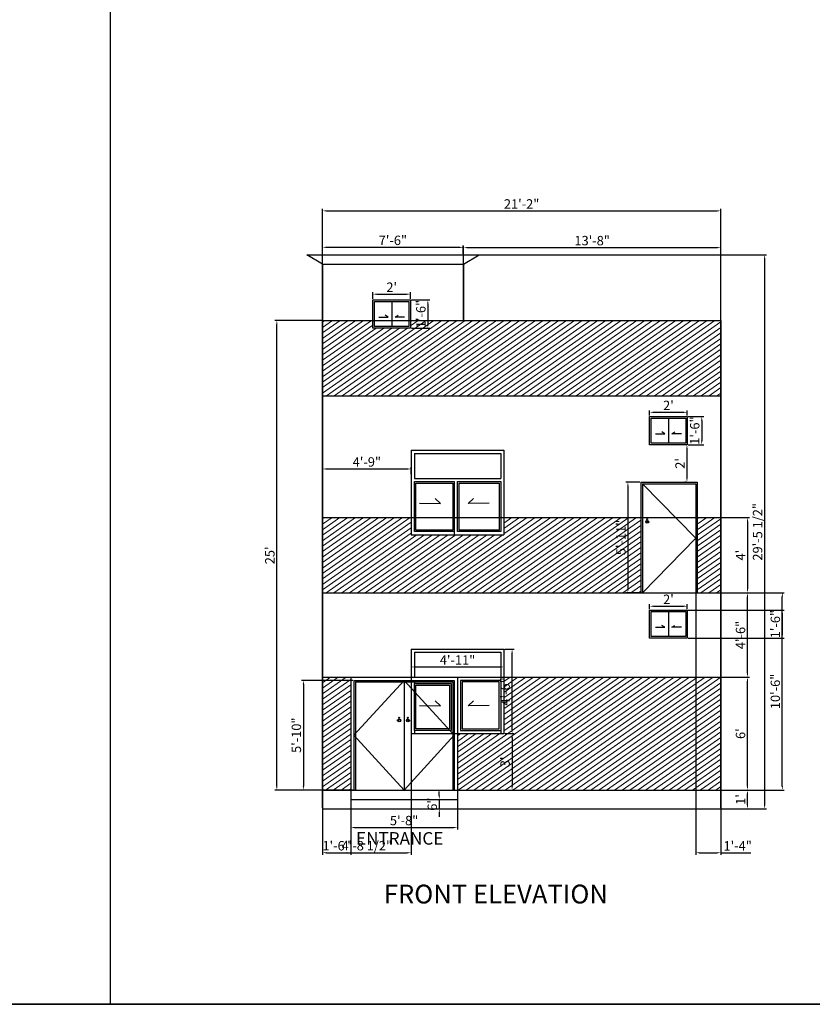
# Model space of a CAD drawing. Units: millimetres. Extents: x 20768 to 23556, y 50760 to 52704.
# Tile 6 of 36: x 21280 to 21786, y 50976 to 51604. Entities that reach past the tile are written whole.
import ezdxf

# ---------------------------------------------------------------- set-up
doc = ezdxf.new("R2010")
doc.units = ezdxf.units.MM
for name, color, linetype, lineweight in [('A-ANNO-DIMS', 2, 'Continuous', 18), ('A-ANNO-TEXT', 7, 'Continuous', 18), ('A-ANNO-TTLB', 7, 'Continuous', 35), ('A-ELEV', 7, 'Continuous', 25), ('A-ELEV-PATT', 8, 'Continuous', 13), ('S-ANNO-DIMS', 2, 'Continuous', 18)]:
    doc.layers.add(name, color=color, linetype=linetype, lineweight=lineweight)
doc.styles.get("Standard").update_dxf_attribs({"font": 'arial.ttf'})
doc.dimstyles.new('ISO-25', dxfattribs={"dimtxt": 6, "dimasz": 2.5, "dimexe": 1.25, "dimexo": 0.625, "dimtad": 1, "dimdec": 0, "dimlunit": 3, "dimtxsty": 'Standard', "dimcen": 2.5, "dimadec": 0, "dimazin": 0, "dimtfac": 1, "dimtdec": 0, "dimtmove": 0, "dimatfit": 3, "dimfxl": 1, "dimarcsym": 0})
pattern_1 = [(215, (166.0957, 0), (1.63899467, -2.34072697), [])]

# ---------------------------------------------------------------- blocks, each defined once
blk = doc.blocks.new('*D146')
at = {"layer": 'A-ANNO-DIMS', "color": 0, "lineweight": -2, "transparency": 16777216}
for p, q in [((21589.53, 51148.5), (21595.42, 51148.5)), ((21594.17, 51146), (21594.17, 51115)), ((21589.53, 51112.5), (21595.42, 51112.5))]:
    blk.add_line(p, q, dxfattribs=at)
at = {"layer": 'A-ANNO-DIMS', "color": 0, "transparency": 16777216}
for points in [[(21593.75, 51146), (21594.59, 51146), (21594.17, 51148.5)], [(21593.75, 51115), (21594.59, 51115), (21594.17, 51112.5)]]:
    blk.add_solid(points, dxfattribs=at)
at = {"layer": 'Defpoints', "color": 0, "transparency": 16777216}
for p in [(21588.91, 51148.5), (21588.91, 51112.5), (21594.17, 51112.5)]:
    blk.add_point(p, dxfattribs=at)
at = {"layer": 'A-ANNO-DIMS', "color": 0, "transparency": 16777216, "insert": (21590.48, 51130.5), "char_height": 6, "attachment_point": 5, "rotation": 90}
blk.add_mtext("3'", dxfattribs=at)
blk = doc.blocks.new('*D147')
at = {"layer": 'A-ANNO-DIMS', "color": 0, "lineweight": -2, "transparency": 16777216}
for p, q in [((21589.53, 51202.4), (21595.42, 51202.4)), ((21594.17, 51151), (21594.17, 51199.9)), ((21589.53, 51148.5), (21595.42, 51148.5))]:
    blk.add_line(p, q, dxfattribs=at)
at = {"layer": 'A-ANNO-DIMS', "color": 0, "transparency": 16777216}
for points in [[(21593.75, 51199.9), (21594.59, 51199.9), (21594.17, 51202.4)], [(21593.75, 51151), (21594.59, 51151), (21594.17, 51148.5)]]:
    blk.add_solid(points, dxfattribs=at)
at = {"layer": 'Defpoints', "color": 0, "transparency": 16777216}
for p in [(21588.91, 51202.4), (21594.17, 51202.4), (21588.91, 51148.5)]:
    blk.add_point(p, dxfattribs=at)
at = {"layer": 'A-ANNO-DIMS', "color": 0, "transparency": 16777216, "insert": (21590.48, 51175.45), "char_height": 6, "attachment_point": 5, "rotation": 90}
blk.add_mtext('4\'-6"', dxfattribs=at)
blk = doc.blocks.new('*D148')
at = {"layer": 'A-ANNO-DIMS', "color": 0, "lineweight": -2, "transparency": 16777216}
for p, q in [((21529.81, 51192.25), (21529.81, 51189.8)), ((21532.31, 51191.05), (21586.41, 51191.05)), ((21588.91, 51192.25), (21588.91, 51189.8))]:
    blk.add_line(p, q, dxfattribs=at)
at = {"layer": 'A-ANNO-DIMS', "color": 0, "transparency": 16777216}
for points in [[(21532.31, 51191.47), (21532.31, 51190.63), (21529.81, 51191.05)], [(21586.41, 51191.47), (21586.41, 51190.63), (21588.91, 51191.05)]]:
    blk.add_solid(points, dxfattribs=at)
at = {"layer": 'Defpoints', "color": 0, "transparency": 16777216}
for p in [(21529.81, 51192.88), (21588.91, 51192.88), (21588.91, 51191.05)]:
    blk.add_point(p, dxfattribs=at)
at = {"layer": 'A-ANNO-DIMS', "color": 0, "transparency": 16777216, "insert": (21559.36, 51194.69), "char_height": 6, "attachment_point": 5}
blk.add_mtext('4\'-11"', dxfattribs=at)
blk = doc.blocks.new('*D149')
at = {"layer": 'A-ANNO-DIMS', "color": 0, "lineweight": -2, "transparency": 16777216}
for p, q in [((21491.21, 51111.87), (21491.21, 51087.33)), ((21559.31, 51111.87), (21559.31, 51087.33)), ((21493.71, 51088.58), (21556.81, 51088.58))]:
    blk.add_line(p, q, dxfattribs=at)
at = {"layer": 'A-ANNO-DIMS', "color": 0, "transparency": 16777216}
for points in [[(21493.71, 51089), (21493.71, 51088.17), (21491.21, 51088.58)], [(21556.81, 51089), (21556.81, 51088.17), (21559.31, 51088.58)]]:
    blk.add_solid(points, dxfattribs=at)
at = {"layer": 'Defpoints', "color": 0, "transparency": 16777216}
for p in [(21491.21, 51112.5), (21559.31, 51112.5), (21559.31, 51088.58)]:
    blk.add_point(p, dxfattribs=at)
at = {"layer": 'A-ANNO-DIMS', "color": 0, "transparency": 16777216, "insert": (21525.26, 51092.27), "char_height": 6, "attachment_point": 5}
blk.add_mtext('5\'-8"', dxfattribs=at)
blk = doc.blocks.new('*D150')
at = {"layer": 'A-ANNO-DIMS', "color": 0, "lineweight": -2, "transparency": 16777216}
for p, q in [((21545.74, 51106.5), (21548.99, 51106.5)), ((21547.74, 51109), (21547.74, 51111.5)), ((21547.74, 51106.5), (21547.74, 51100.5)), ((21545.74, 51100.5), (21548.99, 51100.5)), ((21547.74, 51098), (21547.74, 51095.5))]:
    blk.add_line(p, q, dxfattribs=at)
at = {"layer": 'A-ANNO-DIMS', "color": 0, "transparency": 16777216}
for points in [[(21547.32, 51109), (21548.15, 51109), (21547.74, 51106.5)], [(21547.32, 51098), (21548.15, 51098), (21547.74, 51100.5)]]:
    blk.add_solid(points, dxfattribs=at)
at = {"layer": 'Defpoints', "color": 0, "transparency": 16777216}
for p in [(21545.11, 51106.5), (21545.11, 51100.5), (21547.74, 51100.5)]:
    blk.add_point(p, dxfattribs=at)
at = {"layer": 'A-ANNO-DIMS', "color": 0, "transparency": 16777216, "insert": (21544.05, 51103.5), "char_height": 6, "attachment_point": 5, "rotation": 90}
blk.add_mtext('6"', dxfattribs=at)
blk = doc.blocks.new('*D151')
at = {"layer": 'A-ANNO-DIMS', "color": 0, "lineweight": -2, "transparency": 16777216}
for p, q in [((21681.93, 51228.02), (21681.93, 51231.05)), ((21684.43, 51229.8), (21703.43, 51229.8)), ((21705.93, 51228.02), (21705.93, 51231.05))]:
    blk.add_line(p, q, dxfattribs=at)
at = {"layer": 'A-ANNO-DIMS', "color": 0, "transparency": 16777216}
for points in [[(21684.43, 51230.22), (21684.43, 51229.38), (21681.93, 51229.8)], [(21703.43, 51230.22), (21703.43, 51229.38), (21705.93, 51229.8)]]:
    blk.add_solid(points, dxfattribs=at)
at = {"layer": 'Defpoints', "color": 0, "transparency": 16777216}
for p in [(21681.93, 51227.39), (21705.93, 51229.8), (21705.93, 51227.39)]:
    blk.add_point(p, dxfattribs=at)
at = {"layer": 'A-ANNO-DIMS', "color": 0, "transparency": 16777216, "insert": (21693.93, 51233.44), "char_height": 6, "attachment_point": 5}
blk.add_mtext("2'", dxfattribs=at)
blk = doc.blocks.new('*D152')
at = {"layer": 'A-ANNO-DIMS', "color": 0, "lineweight": -2, "transparency": 16777216}
for p, q in [((21727.93, 51112.5), (21745.63, 51112.5)), ((21744.38, 51103), (21744.38, 51110)), ((21727.93, 51100.5), (21745.63, 51100.5))]:
    blk.add_line(p, q, dxfattribs=at)
at = {"layer": 'A-ANNO-DIMS', "color": 0, "transparency": 16777216}
for points in [[(21743.96, 51110), (21744.79, 51110), (21744.38, 51112.5)], [(21743.96, 51103), (21744.79, 51103), (21744.38, 51100.5)]]:
    blk.add_solid(points, dxfattribs=at)
at = {"layer": 'Defpoints', "color": 0, "transparency": 16777216}
for p in [(21727.31, 51112.5), (21744.38, 51112.5), (21727.31, 51100.5)]:
    blk.add_point(p, dxfattribs=at)
at = {"layer": 'A-ANNO-DIMS', "color": 0, "transparency": 16777216, "insert": (21740.74, 51106.5), "char_height": 6, "attachment_point": 5, "rotation": 90}
blk.add_mtext("1'", dxfattribs=at)
blk = doc.blocks.new('*D153')
at = {"layer": 'A-ANNO-DIMS', "color": 0, "lineweight": -2, "transparency": 16777216}
for p, q in [((21727.93, 51184.5), (21745.63, 51184.5)), ((21744.38, 51115), (21744.38, 51182)), ((21727.93, 51112.5), (21745.63, 51112.5))]:
    blk.add_line(p, q, dxfattribs=at)
at = {"layer": 'A-ANNO-DIMS', "color": 0, "transparency": 16777216}
for points in [[(21743.96, 51182), (21744.79, 51182), (21744.38, 51184.5)], [(21743.96, 51115), (21744.79, 51115), (21744.38, 51112.5)]]:
    blk.add_solid(points, dxfattribs=at)
at = {"layer": 'Defpoints', "color": 0, "transparency": 16777216}
for p in [(21727.31, 51184.5), (21744.38, 51184.5), (21727.31, 51112.5)]:
    blk.add_point(p, dxfattribs=at)
at = {"layer": 'A-ANNO-DIMS', "color": 0, "transparency": 16777216, "insert": (21740.69, 51148.5), "char_height": 6, "attachment_point": 5, "rotation": 90}
blk.add_mtext("6'", dxfattribs=at)
blk = doc.blocks.new('*D154')
at = {"layer": 'A-ANNO-DIMS', "color": 0, "lineweight": -2, "transparency": 16777216}
for p, q in [((21727.93, 51238.4), (21767.84, 51238.4)), ((21766.59, 51115), (21766.59, 51235.9)), ((21727.93, 51112.5), (21767.84, 51112.5))]:
    blk.add_line(p, q, dxfattribs=at)
at = {"layer": 'A-ANNO-DIMS', "color": 0, "transparency": 16777216}
for points in [[(21766.17, 51235.9), (21767, 51235.9), (21766.59, 51238.4)], [(21766.17, 51115), (21767, 51115), (21766.59, 51112.5)]]:
    blk.add_solid(points, dxfattribs=at)
at = {"layer": 'Defpoints', "color": 0, "transparency": 16777216}
for p in [(21727.31, 51238.4), (21766.59, 51238.4), (21727.31, 51112.5)]:
    blk.add_point(p, dxfattribs=at)
at = {"layer": 'A-ANNO-DIMS', "color": 0, "transparency": 16777216, "insert": (21762.9, 51175.45), "char_height": 6, "attachment_point": 5, "rotation": 90}
blk.add_mtext('10\'-6"', dxfattribs=at)
blk = doc.blocks.new('*D142')
at = {"layer": 'A-ANNO-DIMS', "color": 0, "lineweight": -2, "transparency": 16777216}
for p, q in [((21727.93, 51238.4), (21745.63, 51238.4)), ((21744.38, 51187), (21744.38, 51235.9)), ((21727.93, 51184.5), (21745.63, 51184.5))]:
    blk.add_line(p, q, dxfattribs=at)
at = {"layer": 'A-ANNO-DIMS', "color": 0, "transparency": 16777216}
for points in [[(21743.96, 51235.9), (21744.79, 51235.9), (21744.38, 51238.4)], [(21743.96, 51187), (21744.79, 51187), (21744.38, 51184.5)]]:
    blk.add_solid(points, dxfattribs=at)
at = {"layer": 'Defpoints', "color": 0, "transparency": 16777216}
for p in [(21727.31, 51238.4), (21744.38, 51238.4), (21727.31, 51184.5)]:
    blk.add_point(p, dxfattribs=at)
at = {"layer": 'A-ANNO-DIMS', "color": 0, "transparency": 16777216, "insert": (21740.69, 51211.45), "char_height": 6, "attachment_point": 5, "rotation": 90}
blk.add_mtext('4\'-6"', dxfattribs=at)
blk = doc.blocks.new('*D155')
at = {"layer": 'A-ANNO-DIMS', "color": 0, "lineweight": -2, "transparency": 16777216}
for p, q in [((21706.56, 51227.39), (21767.84, 51227.39)), ((21766.59, 51224.89), (21766.59, 51211.89)), ((21706.56, 51209.39), (21767.84, 51209.39))]:
    blk.add_line(p, q, dxfattribs=at)
at = {"layer": 'A-ANNO-DIMS', "color": 0, "transparency": 16777216}
for points in [[(21766.17, 51224.89), (21767, 51224.89), (21766.59, 51227.39)], [(21766.17, 51211.89), (21767, 51211.89), (21766.59, 51209.39)]]:
    blk.add_solid(points, dxfattribs=at)
at = {"layer": 'Defpoints', "color": 0, "transparency": 16777216}
for p in [(21705.93, 51227.39), (21705.93, 51209.39), (21766.59, 51209.39)]:
    blk.add_point(p, dxfattribs=at)
at = {"layer": 'A-ANNO-DIMS', "color": 0, "transparency": 16777216, "insert": (21762.9, 51218.39), "char_height": 6, "attachment_point": 5, "rotation": 90}
blk.add_mtext('1\'-6"', dxfattribs=at)
blk = doc.blocks.new('*D156')
at = {"layer": 'A-ANNO-DIMS', "color": 0, "lineweight": -2, "transparency": 16777216}
for p, q in [((21727.93, 51286.4), (21745.63, 51286.4)), ((21744.38, 51283.9), (21744.38, 51240.9)), ((21727.93, 51238.4), (21745.63, 51238.4))]:
    blk.add_line(p, q, dxfattribs=at)
at = {"layer": 'A-ANNO-DIMS', "color": 0, "transparency": 16777216}
for points in [[(21743.96, 51283.9), (21744.79, 51283.9), (21744.38, 51286.4)], [(21743.96, 51240.9), (21744.79, 51240.9), (21744.38, 51238.4)]]:
    blk.add_solid(points, dxfattribs=at)
at = {"layer": 'Defpoints', "color": 0, "transparency": 16777216}
for p in [(21727.31, 51286.4), (21727.31, 51238.4), (21744.38, 51238.4)]:
    blk.add_point(p, dxfattribs=at)
at = {"layer": 'A-ANNO-DIMS', "color": 0, "transparency": 16777216, "insert": (21740.75, 51262.4), "char_height": 6, "attachment_point": 5, "rotation": 90}
blk.add_mtext("4'", dxfattribs=at)
blk = doc.blocks.new('*D157')
at = {"layer": 'A-ANNO-DIMS', "color": 0, "lineweight": -2, "transparency": 16777216}
for p, q in [((21675.68, 51309), (21666.81, 51309)), ((21668.06, 51306.5), (21668.06, 51240.9)), ((21675.68, 51238.4), (21666.81, 51238.4))]:
    blk.add_line(p, q, dxfattribs=at)
at = {"layer": 'A-ANNO-DIMS', "color": 0, "transparency": 16777216}
for points in [[(21667.64, 51306.5), (21668.47, 51306.5), (21668.06, 51309)], [(21667.64, 51240.9), (21668.47, 51240.9), (21668.06, 51238.4)]]:
    blk.add_solid(points, dxfattribs=at)
at = {"layer": 'Defpoints', "color": 0, "transparency": 16777216}
for p in [(21676.31, 51309), (21668.06, 51238.4), (21676.31, 51238.4)]:
    blk.add_point(p, dxfattribs=at)
at = {"layer": 'A-ANNO-DIMS', "color": 0, "transparency": 16777216, "insert": (21664.37, 51273.7), "char_height": 6, "attachment_point": 5, "rotation": 90}
blk.add_mtext('5\'-11"', dxfattribs=at)
blk = doc.blocks.new('*D158')
at = {"layer": 'A-ANNO-DIMS', "color": 0, "lineweight": -2, "transparency": 16777216}
for p, q in [((21705.31, 51332.9), (21704.48, 51332.9)), ((21705.73, 51330.4), (21705.73, 51311.5)), ((21705.31, 51309), (21704.48, 51309))]:
    blk.add_line(p, q, dxfattribs=at)
at = {"layer": 'A-ANNO-DIMS', "color": 0, "transparency": 16777216}
for points in [[(21705.31, 51330.4), (21706.14, 51330.4), (21705.73, 51332.9)], [(21705.31, 51311.5), (21706.14, 51311.5), (21705.73, 51309)]]:
    blk.add_solid(points, dxfattribs=at)
at = {"layer": 'Defpoints', "color": 0, "transparency": 16777216}
for p in [(21705.93, 51332.9), (21705.73, 51309), (21705.93, 51309)]:
    blk.add_point(p, dxfattribs=at)
at = {"layer": 'A-ANNO-DIMS', "color": 0, "transparency": 16777216, "insert": (21702.09, 51320.95), "char_height": 6, "attachment_point": 5, "rotation": 90}
blk.add_mtext("2'", dxfattribs=at)
blk = doc.blocks.new('*D159')
at = {"layer": 'A-ANNO-DIMS', "color": 0, "lineweight": -2, "transparency": 16777216}
for p, q in [((21681.93, 51351.52), (21681.93, 51354.8)), ((21684.43, 51353.55), (21703.43, 51353.55)), ((21705.93, 51351.52), (21705.93, 51354.8))]:
    blk.add_line(p, q, dxfattribs=at)
at = {"layer": 'A-ANNO-DIMS', "color": 0, "transparency": 16777216}
for points in [[(21684.43, 51353.96), (21684.43, 51353.13), (21681.93, 51353.55)], [(21703.43, 51353.96), (21703.43, 51353.13), (21705.93, 51353.55)]]:
    blk.add_solid(points, dxfattribs=at)
at = {"layer": 'Defpoints', "color": 0, "transparency": 16777216}
for p in [(21705.93, 51353.55), (21681.93, 51350.9), (21705.93, 51350.9)]:
    blk.add_point(p, dxfattribs=at)
at = {"layer": 'A-ANNO-DIMS', "color": 0, "transparency": 16777216, "insert": (21693.93, 51357.19), "char_height": 6, "attachment_point": 5}
blk.add_mtext("2'", dxfattribs=at)
blk = doc.blocks.new('*D143')
at = {"layer": 'A-ANNO-DIMS', "color": 0, "lineweight": -2, "transparency": 16777216}
for p, q in [((21706.56, 51350.9), (21716.42, 51350.9)), ((21715.17, 51348.4), (21715.17, 51335.4)), ((21706.56, 51332.9), (21716.42, 51332.9))]:
    blk.add_line(p, q, dxfattribs=at)
at = {"layer": 'A-ANNO-DIMS', "color": 0, "transparency": 16777216}
for points in [[(21714.75, 51348.4), (21715.58, 51348.4), (21715.17, 51350.9)], [(21714.75, 51335.4), (21715.58, 51335.4), (21715.17, 51332.9)]]:
    blk.add_solid(points, dxfattribs=at)
at = {"layer": 'Defpoints', "color": 0, "transparency": 16777216}
for p in [(21705.93, 51350.9), (21705.93, 51332.9), (21715.17, 51332.9)]:
    blk.add_point(p, dxfattribs=at)
at = {"layer": 'A-ANNO-DIMS', "color": 0, "transparency": 16777216, "insert": (21711.48, 51341.9), "char_height": 6, "attachment_point": 5, "rotation": 90}
blk.add_mtext('1\'-6"', dxfattribs=at)
blk = doc.blocks.new('*D160')
at = {"layer": 'A-ANNO-DIMS', "color": 0, "lineweight": -2, "transparency": 16777216}
for p, q in [((21473.21, 51314.02), (21473.21, 51318.65)), ((21475.71, 51317.4), (21527.31, 51317.4)), ((21529.81, 51314.02), (21529.81, 51318.65))]:
    blk.add_line(p, q, dxfattribs=at)
at = {"layer": 'A-ANNO-DIMS', "color": 0, "transparency": 16777216}
for points in [[(21475.71, 51317.82), (21475.71, 51316.99), (21473.21, 51317.4)], [(21527.31, 51317.82), (21527.31, 51316.99), (21529.81, 51317.4)]]:
    blk.add_solid(points, dxfattribs=at)
at = {"layer": 'Defpoints', "color": 0, "transparency": 16777216}
for p in [(21529.81, 51317.4), (21473.21, 51313.39), (21529.81, 51313.39)]:
    blk.add_point(p, dxfattribs=at)
at = {"layer": 'A-ANNO-DIMS', "color": 0, "transparency": 16777216, "insert": (21501.51, 51321.09), "char_height": 6, "attachment_point": 5}
blk.add_mtext('4\'-9"', dxfattribs=at)
blk = doc.blocks.new('*D161')
at = {"layer": 'A-ANNO-DIMS', "color": 0, "lineweight": -2, "transparency": 16777216}
for p, q in [((21492.58, 51182.5), (21459.76, 51182.5)), ((21461.01, 51180), (21461.01, 51115)), ((21492.58, 51112.5), (21459.76, 51112.5))]:
    blk.add_line(p, q, dxfattribs=at)
at = {"layer": 'A-ANNO-DIMS', "color": 0, "transparency": 16777216}
for points in [[(21460.6, 51180), (21461.43, 51180), (21461.01, 51182.5)], [(21460.6, 51115), (21461.43, 51115), (21461.01, 51112.5)]]:
    blk.add_solid(points, dxfattribs=at)
at = {"layer": 'Defpoints', "color": 0, "transparency": 16777216}
for p in [(21493.21, 51182.5), (21461.01, 51112.5), (21493.21, 51112.5)]:
    blk.add_point(p, dxfattribs=at)
at = {"layer": 'A-ANNO-DIMS', "color": 0, "transparency": 16777216, "insert": (21457.32, 51147.5), "char_height": 6, "attachment_point": 5, "rotation": 90}
blk.add_mtext('5\'-10"', dxfattribs=at)
blk = doc.blocks.new('*D162')
at = {"layer": 'A-ANNO-DIMS', "color": 0, "lineweight": -2, "transparency": 16777216}
for p, q in [((21472.58, 51412.1), (21442.83, 51412.1)), ((21444.08, 51114.96), (21444.08, 51409.6)), ((21472.58, 51112.46), (21442.83, 51112.46))]:
    blk.add_line(p, q, dxfattribs=at)
at = {"layer": 'A-ANNO-DIMS', "color": 0, "transparency": 16777216}
for points in [[(21443.67, 51409.6), (21444.5, 51409.6), (21444.08, 51412.1)], [(21443.67, 51114.96), (21444.5, 51114.96), (21444.08, 51112.46)]]:
    blk.add_solid(points, dxfattribs=at)
at = {"layer": 'Defpoints', "color": 0, "transparency": 16777216}
for p in [(21444.08, 51412.1), (21473.21, 51412.1), (21473.21, 51112.46)]:
    blk.add_point(p, dxfattribs=at)
at = {"layer": 'A-ANNO-DIMS', "color": 0, "transparency": 16777216, "insert": (21440.39, 51262.28), "char_height": 6, "attachment_point": 5, "rotation": 90}
blk.add_mtext("25'", dxfattribs=at)
blk = doc.blocks.new('*D163')
at = {"layer": 'A-ANNO-DIMS', "color": 0, "lineweight": -2, "transparency": 16777216}
for p, q in [((21473.21, 51454.72), (21473.21, 51460.08)), ((21475.71, 51458.83), (21560.54, 51458.83)), ((21563.04, 51454.72), (21563.04, 51460.08))]:
    blk.add_line(p, q, dxfattribs=at)
at = {"layer": 'A-ANNO-DIMS', "color": 0, "transparency": 16777216}
for points in [[(21475.71, 51459.25), (21475.71, 51458.42), (21473.21, 51458.83)], [(21560.54, 51459.25), (21560.54, 51458.42), (21563.04, 51458.83)]]:
    blk.add_solid(points, dxfattribs=at)
at = {"layer": 'Defpoints', "color": 0, "transparency": 16777216}
for p in [(21563.04, 51458.83), (21473.21, 51454.1), (21563.04, 51454.1)]:
    blk.add_point(p, dxfattribs=at)
at = {"layer": 'A-ANNO-DIMS', "color": 0, "transparency": 16777216, "insert": (21518.12, 51462.52), "char_height": 6, "attachment_point": 5}
blk.add_mtext('7\'-6"', dxfattribs=at)
blk = doc.blocks.new('*D164')
at = {"layer": 'A-ANNO-DIMS', "color": 0, "lineweight": -2, "transparency": 16777216}
for p, q in [((21505.36, 51425.88), (21505.36, 51430.21)), ((21507.86, 51428.96), (21526.86, 51428.96)), ((21529.36, 51425.88), (21529.36, 51430.21))]:
    blk.add_line(p, q, dxfattribs=at)
at = {"layer": 'A-ANNO-DIMS', "color": 0, "transparency": 16777216}
for points in [[(21507.86, 51429.38), (21507.86, 51428.54), (21505.36, 51428.96)], [(21526.86, 51429.38), (21526.86, 51428.54), (21529.36, 51428.96)]]:
    blk.add_solid(points, dxfattribs=at)
at = {"layer": 'Defpoints', "color": 0, "transparency": 16777216}
for p in [(21529.36, 51428.96), (21505.36, 51425.25), (21529.36, 51425.25)]:
    blk.add_point(p, dxfattribs=at)
at = {"layer": 'A-ANNO-DIMS', "color": 0, "transparency": 16777216, "insert": (21517.36, 51432.6), "char_height": 6, "attachment_point": 5}
blk.add_mtext("2'", dxfattribs=at)
blk = doc.blocks.new('*D144')
at = {"layer": 'A-ANNO-DIMS', "color": 0, "lineweight": -2, "transparency": 16777216}
for p, q in [((21529.98, 51425.25), (21541.69, 51425.25)), ((21540.44, 51422.75), (21540.44, 51409.75)), ((21529.98, 51407.25), (21541.69, 51407.25))]:
    blk.add_line(p, q, dxfattribs=at)
at = {"layer": 'A-ANNO-DIMS', "color": 0, "transparency": 16777216}
for points in [[(21540.02, 51422.75), (21540.85, 51422.75), (21540.44, 51425.25)], [(21540.02, 51409.75), (21540.85, 51409.75), (21540.44, 51407.25)]]:
    blk.add_solid(points, dxfattribs=at)
at = {"layer": 'Defpoints', "color": 0, "transparency": 16777216}
for p in [(21529.36, 51425.25), (21529.36, 51407.25), (21540.44, 51407.25)]:
    blk.add_point(p, dxfattribs=at)
at = {"layer": 'A-ANNO-DIMS', "color": 0, "transparency": 16777216, "insert": (21536.75, 51416.25), "char_height": 6, "attachment_point": 5, "rotation": 90}
blk.add_mtext('1\'-6"', dxfattribs=at)
blk = doc.blocks.new('*D145')
at = {"layer": 'A-ANNO-DIMS', "color": 0, "lineweight": -2, "transparency": 16777216}
for p, q in [((21563.21, 51412.72), (21563.21, 51459.88)), ((21565.71, 51458.63), (21724.81, 51458.63)), ((21727.31, 51412.72), (21727.31, 51459.88))]:
    blk.add_line(p, q, dxfattribs=at)
at = {"layer": 'A-ANNO-DIMS', "color": 0, "transparency": 16777216}
for points in [[(21565.71, 51459.04), (21565.71, 51458.21), (21563.21, 51458.63)], [(21724.81, 51459.04), (21724.81, 51458.21), (21727.31, 51458.63)]]:
    blk.add_solid(points, dxfattribs=at)
at = {"layer": 'Defpoints', "color": 0, "transparency": 16777216}
for p in [(21727.31, 51458.63), (21563.21, 51412.1), (21727.31, 51412.1)]:
    blk.add_point(p, dxfattribs=at)
at = {"layer": 'A-ANNO-DIMS', "color": 0, "transparency": 16777216, "insert": (21645.26, 51462.32), "char_height": 6, "attachment_point": 5}
blk.add_mtext('13\'-8"', dxfattribs=at)
blk = doc.blocks.new('*D232')
at = {"layer": 'Defpoints', "color": 0, "transparency": 16777216}
for p in [(21727.31, 51482.1), (21473.21, 51100.5), (21727.31, 51100.5)]:
    blk.add_point(p, dxfattribs=at)
at = {"layer": 'S-ANNO-DIMS', "color": 0, "lineweight": -2, "transparency": 16777216}
for p, q in [((21473.21, 51101.12), (21473.21, 51483.35)), ((21475.71, 51482.1), (21724.81, 51482.1)), ((21727.31, 51101.12), (21727.31, 51483.35))]:
    blk.add_line(p, q, dxfattribs=at)
at = {"layer": 'S-ANNO-DIMS', "color": 0, "transparency": 16777216}
for points in [[(21475.71, 51482.51), (21475.71, 51481.68), (21473.21, 51482.1)], [(21724.81, 51482.51), (21724.81, 51481.68), (21727.31, 51482.1)]]:
    blk.add_solid(points, dxfattribs=at)
at = {"layer": 'S-ANNO-DIMS', "color": 0, "transparency": 16777216, "insert": (21600.26, 51485.74), "char_height": 6, "attachment_point": 5}
blk.add_mtext('21\'-2"', dxfattribs=at)
blk = doc.blocks.new('*D233')
at = {"layer": 'Defpoints', "color": 0, "transparency": 16777216}
for p in [(21463.23, 51454.1), (21473.21, 51100.5), (21755.31, 51100.5)]:
    blk.add_point(p, dxfattribs=at)
at = {"layer": 'S-ANNO-DIMS', "color": 0, "lineweight": -2, "transparency": 16777216}
for p, q in [((21463.86, 51454.1), (21756.56, 51454.1)), ((21755.31, 51451.6), (21755.31, 51103)), ((21473.83, 51100.5), (21756.56, 51100.5))]:
    blk.add_line(p, q, dxfattribs=at)
at = {"layer": 'S-ANNO-DIMS', "color": 0, "transparency": 16777216}
for points in [[(21754.89, 51451.6), (21755.72, 51451.6), (21755.31, 51454.1)], [(21754.89, 51103), (21755.72, 51103), (21755.31, 51100.5)]]:
    blk.add_solid(points, dxfattribs=at)
at = {"layer": 'S-ANNO-DIMS', "color": 0, "transparency": 16777216, "insert": (21751.58, 51277.3), "char_height": 6, "attachment_point": 5, "rotation": 90}
blk.add_mtext('29\'-5 1/2"', dxfattribs=at)
blk = doc.blocks.new('*D234')
at = {"layer": 'Defpoints', "color": 0, "transparency": 16777216}
for p in [(21491.21, 51106.5), (21473.21, 51100.5), (21491.21, 51072.5)]:
    blk.add_point(p, dxfattribs=at)
at = {"layer": 'S-ANNO-DIMS', "color": 0, "lineweight": -2, "transparency": 16777216}
for p, q in [((21491.21, 51105.87), (21491.21, 51071.25)), ((21473.21, 51099.87), (21473.21, 51071.25)), ((21475.71, 51072.5), (21488.71, 51072.5))]:
    blk.add_line(p, q, dxfattribs=at)
at = {"layer": 'S-ANNO-DIMS', "color": 0, "transparency": 16777216}
for points in [[(21475.71, 51072.91), (21475.71, 51072.08), (21473.21, 51072.5)], [(21488.71, 51072.91), (21488.71, 51072.08), (21491.21, 51072.5)]]:
    blk.add_solid(points, dxfattribs=at)
at = {"layer": 'S-ANNO-DIMS', "color": 0, "transparency": 16777216, "insert": (21482.21, 51076.19), "char_height": 6, "attachment_point": 5}
blk.add_mtext('1\'-6"', dxfattribs=at)
blk = doc.blocks.new('*D235')
at = {"layer": 'Defpoints', "color": 0, "transparency": 16777216}
for p in [(21711.31, 51238.4), (21727.31, 51238.4), (21727.31, 51072.5)]:
    blk.add_point(p, dxfattribs=at)
at = {"layer": 'S-ANNO-DIMS', "color": 0, "lineweight": -2, "transparency": 16777216}
for p, q in [((21711.31, 51237.77), (21711.31, 51071.25)), ((21727.31, 51237.77), (21727.31, 51071.25)), ((21713.81, 51072.5), (21724.81, 51072.5)), ((21727.31, 51072.5), (21746.44, 51072.5))]:
    blk.add_line(p, q, dxfattribs=at)
at = {"layer": 'S-ANNO-DIMS', "color": 0, "transparency": 16777216}
for points in [[(21713.81, 51072.91), (21713.81, 51072.08), (21711.31, 51072.5)], [(21724.81, 51072.91), (21724.81, 51072.08), (21727.31, 51072.5)]]:
    blk.add_solid(points, dxfattribs=at)
at = {"layer": 'S-ANNO-DIMS', "color": 0, "transparency": 16777216, "insert": (21738.12, 51076.14), "char_height": 6, "attachment_point": 5}
blk.add_mtext('1\'-4"', dxfattribs=at)
blk = doc.blocks.new('*D236')
at = {"layer": 'Defpoints', "color": 0, "transparency": 16777216}
for p in [(21529.81, 51202.4), (21473.21, 51184.5), (21529.81, 51072.5)]:
    blk.add_point(p, dxfattribs=at)
at = {"layer": 'S-ANNO-DIMS', "color": 0, "lineweight": -2, "transparency": 16777216}
for p, q in [((21529.81, 51201.77), (21529.81, 51071.25)), ((21473.21, 51183.87), (21473.21, 51071.25)), ((21475.71, 51072.5), (21527.31, 51072.5))]:
    blk.add_line(p, q, dxfattribs=at)
at = {"layer": 'S-ANNO-DIMS', "color": 0, "transparency": 16777216}
for points in [[(21475.71, 51072.91), (21475.71, 51072.08), (21473.21, 51072.5)], [(21527.31, 51072.91), (21527.31, 51072.08), (21529.81, 51072.5)]]:
    blk.add_solid(points, dxfattribs=at)
at = {"layer": 'S-ANNO-DIMS', "color": 0, "transparency": 16777216, "insert": (21501.51, 51076.23), "char_height": 6, "attachment_point": 5}
blk.add_mtext('4\'-8 1/2"', dxfattribs=at)

msp = doc.modelspace()

# ---------------------------------------------------------------- hatches: boundary and pattern name
at = {"layer": 'A-ELEV-PATT'}
h = msp.add_hatch(dxfattribs=at)
h.set_pattern_fill('ANSI31', color=256, scale=0.9, angle=170)
h.set_pattern_definition(pattern_1)
h.paths.add_polyline_path([(21727.31, 51412.1), (21529.36, 51412.1), (21529.36, 51407.25), (21505.36, 51407.25), (21505.36, 51412.1), (21473.21, 51412.1), (21473.21, 51364.1), (21727.31, 51364.1)])
h = msp.add_hatch(dxfattribs=at)
h.set_pattern_fill('ANSI31', color=256, scale=0.9, angle=170)
h.set_pattern_definition(pattern_1)
h.paths.add_polyline_path([(21676.31, 51286.4), (21588.91, 51286.4), (21588.91, 51275.39), (21529.81, 51275.39), (21529.81, 51286.4), (21473.21, 51286.4), (21473.21, 51238.4), (21676.31, 51238.4)])
h = msp.add_hatch(dxfattribs=at)
h.set_pattern_fill('ANSI31', color=256, scale=0.9, angle=170)
h.set_pattern_definition(pattern_1)
h.paths.add_polyline_path([(21727.31, 51286.4), (21712.31, 51286.4), (21712.31, 51238.4), (21727.31, 51238.4)])
h = msp.add_hatch(dxfattribs=at)
h.set_pattern_fill('ANSI31', color=256, scale=0.9, angle=170)
h.set_pattern_definition(pattern_1)
h.paths.add_polyline_path([(21491.21, 51184.5), (21473.21, 51184.5), (21473.21, 51112.5), (21491.21, 51112.5)])
h = msp.add_hatch(dxfattribs=at)
h.set_pattern_fill('ANSI31', color=256, scale=0.9, angle=170)
h.set_pattern_definition(pattern_1)
h.paths.add_polyline_path([(21727.31, 51184.5), (21588.91, 51184.5), (21588.91, 51148.5), (21559.31, 51148.5), (21559.31, 51112.5), (21727.31, 51112.5)])

# ---------------------------------------------------------------- linework, layer by layer
at = {"layer": 'A-ANNO-TTLB'}
msp.add_line((20768.14, 50975.78), (22719.7, 50975.78), dxfattribs=at)
at = {"layer": 'A-ELEV'}
for p, q in [((21337.76, 51623.53), (21337.76, 50975.78)), ((21463.23, 51454.1), (21573.18, 51454.1)), ((21473.21, 51448.1), (21463.23, 51454.1)), ((21563.21, 51448.1), (21573.18, 51454.1)), ((21473.21, 51448.1), (21473.21, 51100.5)), ((21473.21, 51448.1), (21563.21, 51448.1)), ((21563.21, 51448.1), (21563.21, 51412.1)), ((21517.36, 51424.25), (21517.36, 51408.25)), ((21515.11, 51414.25), (21513.21, 51415.46)), ((21519.61, 51414.25), (21521.5, 51415.46)), ((21473.21, 51412.1), (21727.31, 51412.1)), ((21509.13, 51414.25), (21515.11, 51414.25)), ((21525.59, 51414.25), (21519.61, 51414.25)), ((21727.31, 51412.1), (21727.31, 51100.5)), ((21473.21, 51364.1), (21727.31, 51364.1)), ((21693.93, 51349.9), (21693.93, 51333.9)), ((21685.7, 51339.89), (21691.68, 51339.89)), ((21691.68, 51339.89), (21689.79, 51341.1)), ((21696.18, 51339.89), (21698.08, 51341.1)), ((21702.16, 51339.89), (21696.18, 51339.89)), ((21529.81, 51329.29), (21529.81, 51275.39)), ((21529.81, 51329.29), (21588.91, 51329.29)), ((21531.81, 51327.29), (21531.81, 51311.39)), ((21531.81, 51327.29), (21586.91, 51327.29)), ((21586.91, 51327.29), (21586.91, 51311.39)), ((21588.91, 51329.29), (21588.91, 51275.39)), ((21531.81, 51311.39), (21586.91, 51311.39)), ((21531.81, 51309.39), (21557.31, 51309.39)), ((21531.81, 51277.39), (21531.81, 51309.39)), ((21532.81, 51308.39), (21556.31, 51308.39)), ((21532.81, 51278.39), (21532.81, 51308.39)), ((21556.31, 51308.39), (21556.31, 51278.39)), ((21557.31, 51309.39), (21557.31, 51275.39)), ((21676.31, 51309), (21676.31, 51238.4)), ((21676.31, 51309), (21712.31, 51309)), ((21677.31, 51308), (21677.31, 51238.4)), ((21677.31, 51308), (21711.31, 51308)), ((21677.31, 51308), (21711.31, 51273.2)), ((21711.31, 51308), (21711.31, 51238.4)), ((21712.31, 51309), (21712.31, 51238.4)), ((21535.03, 51295.65), (21548.5, 51295.34)), ((21548.5, 51295.34), (21545, 51298.51)), ((21566.11, 51295.34), (21569.62, 51298.51)), ((21579.59, 51295.65), (21566.11, 51295.34)), ((21473.21, 51286.4), (21727.31, 51286.4)), ((21680.29, 51283.62), (21680.29, 51285.14)), ((21680.29, 51283.62), (21681.8, 51283.62)), ((21680.4, 51283.69), (21680.4, 51285.14)), ((21680.4, 51283.69), (21681.8, 51283.69)), ((21681.8, 51283.69), (21681.8, 51283.62)), ((21557.31, 51277.39), (21531.81, 51277.39)), ((21556.31, 51278.39), (21532.81, 51278.39)), ((21529.81, 51275.39), (21588.91, 51275.39)), ((21711.31, 51273.2), (21677.31, 51238.4)), ((21473.21, 51238.4), (21727.31, 51238.4)), ((21693.93, 51226.39), (21693.93, 51210.39)), ((21685.7, 51216.39), (21691.68, 51216.39)), ((21691.68, 51216.39), (21689.79, 51217.6)), ((21696.18, 51216.39), (21698.08, 51217.6)), ((21702.16, 51216.39), (21696.18, 51216.39)), ((21529.81, 51202.4), (21529.81, 51148.5)), ((21529.81, 51202.4), (21588.91, 51202.4)), ((21588.91, 51202.4), (21588.91, 51148.5)), ((21531.81, 51200.4), (21531.81, 51184.5)), ((21531.81, 51200.4), (21586.91, 51200.4)), ((21586.91, 51200.4), (21586.91, 51184.5)), ((21473.21, 51184.5), (21727.31, 51184.5)), ((21491.21, 51184.5), (21491.21, 51100.5)), ((21493.21, 51182.5), (21493.21, 51112.5)), ((21493.21, 51182.5), (21557.31, 51182.5)), ((21525.26, 51182.5), (21493.21, 51147.5)), ((21525.26, 51182.5), (21525.26, 51112.5)), ((21557.31, 51147.5), (21525.26, 51182.5)), ((21531.81, 51182.5), (21531.81, 51180.5)), ((21557.31, 51182.5), (21557.31, 51112.5)), ((21559.31, 51184.5), (21559.31, 51100.5)), ((21586.91, 51182.5), (21586.91, 51150.5)), ((21494.21, 51181.5), (21494.21, 51112.5)), ((21494.21, 51181.5), (21556.31, 51181.5)), ((21556.31, 51181.5), (21556.31, 51112.5)), ((21548.5, 51166.18), (21545, 51169.35)), ((21566.11, 51166.18), (21569.62, 51169.35)), ((21535.03, 51166.5), (21548.5, 51166.18)), ((21579.59, 51166.5), (21566.11, 51166.18)), ((21522.11, 51156.96), (21520.71, 51156.96)), ((21522.22, 51156.89), (21520.71, 51156.89)), ((21522.11, 51156.96), (21522.11, 51158.41)), ((21522.22, 51156.89), (21522.22, 51158.41)), ((21527.62, 51156.89), (21527.62, 51158.41)), ((21527.62, 51156.89), (21529.13, 51156.89)), ((21527.73, 51156.96), (21527.73, 51158.41)), ((21527.73, 51156.96), (21529.13, 51156.96)), ((21529.13, 51156.96), (21529.13, 51156.89)), ((21531.81, 51150.5), (21531.81, 51148.5)), ((21586.91, 51150.5), (21586.91, 51148.5)), ((21493.21, 51147.5), (21525.26, 51112.5)), ((21525.26, 51112.5), (21557.31, 51147.5)), ((21529.81, 51148.5), (21588.91, 51148.5)), ((21473.21, 51112.5), (21727.31, 51112.5)), ((21491.21, 51106.5), (21559.31, 51106.5)), ((21473.21, 51100.5), (21727.31, 51100.5))]:
    msp.add_line(p, q, dxfattribs=at)
for points in [[(21529.36, 51407.25), (21505.36, 51407.25), (21505.36, 51425.25), (21529.36, 51425.25)], [(21528.36, 51408.25), (21506.36, 51408.25), (21506.36, 51424.25), (21528.36, 51424.25)], [(21705.93, 51332.9), (21681.93, 51332.9), (21681.93, 51350.9), (21705.93, 51350.9)], [(21704.93, 51333.9), (21682.93, 51333.9), (21682.93, 51349.9), (21704.93, 51349.9)], [(21559.31, 51277.39), (21559.31, 51309.39), (21586.91, 51309.39), (21586.91, 51277.39)], [(21560.31, 51278.39), (21560.31, 51308.39), (21585.91, 51308.39), (21585.91, 51278.39)], [(21705.93, 51209.39), (21681.93, 51209.39), (21681.93, 51227.39), (21705.93, 51227.39)], [(21704.93, 51210.39), (21682.93, 51210.39), (21682.93, 51226.39), (21704.93, 51226.39)], [(21531.81, 51180.5), (21555.31, 51180.5), (21555.31, 51150.5), (21531.81, 51150.5)], [(21532.81, 51179.5), (21554.31, 51179.5), (21554.31, 51151.5), (21532.81, 51151.5)], [(21562.31, 51181.5), (21562.31, 51151.5), (21585.91, 51151.5), (21585.91, 51181.5)]]:
    msp.add_lwpolyline(points, close=True, dxfattribs=at)
msp.add_lwpolyline([(21586.91, 51182.5), (21561.31, 51182.5), (21561.31, 51150.5), (21586.91, 51150.5)], dxfattribs=at)
for centre, radius in [((21680.29, 51283.69), 0.877), ((21680.34, 51285.4), 0.272), ((21522.22, 51156.96), 0.877), ((21522.17, 51158.67), 0.272), ((21527.62, 51156.96), 0.877), ((21527.67, 51158.67), 0.272)]:
    msp.add_circle(centre, radius, dxfattribs=at)

# ---------------------------------------------------------------- texts
at = {"layer": 'A-ANNO-TEXT', "attachment_point": 1}
for s, width, insert, char_height in [('ENTRANCE', 27.5349, (21494.61, 51085.65), 8), ('  FRONT ELEVATION', 241.5904, (21504.97, 51052.13), 12)]:
    msp.add_mtext_dynamic_manual_height_columns(s, width=width, gutter_width=12.5, heights=[0], dxfattribs=dict(at, insert=insert, char_height=char_height))

# ---------------------------------------------------------------- dimensions: what is measured, and where the dimension line sits
at = {"layer": 'A-ANNO-DIMS'}
for base, p1, p2, picture, middle in [((21563.04, 51458.83), (21473.21, 51454.1), (21563.04, 51454.1), '*D163', (21518.12, 51462.52)), ((21727.31, 51458.63), (21563.21, 51412.1), (21727.31, 51412.1), '*D145', (21645.26, 51462.32)), ((21529.36, 51428.96), (21505.36, 51425.25), (21529.36, 51425.25), '*D164', (21517.36, 51432.6)), ((21705.93, 51353.55), (21681.93, 51350.9), (21705.93, 51350.9), '*D159', (21693.93, 51357.19)), ((21529.81, 51317.4), (21473.21, 51313.39), (21529.81, 51313.39), '*D160', (21501.51, 51321.09)), ((21705.93, 51229.8), (21681.93, 51227.39), (21705.93, 51227.39), '*D151', (21693.93, 51233.44)), ((21588.91, 51191.05), (21529.81, 51192.88), (21588.91, 51192.88), '*D148', (21559.36, 51194.69)), ((21559.31, 51088.58), (21491.21, 51112.5), (21559.31, 51112.5), '*D149', (21525.26, 51092.27))]:
    dim = msp.add_linear_dim(base=base, p1=p1, p2=p2, dimstyle='ISO-25', override={"dimclrd": 0, "dimclre": 0, "dimclrt": 0}, dxfattribs=at)
    dim.commit()
    dim.dimension.update_dxf_attribs({"geometry": picture, "text_midpoint": middle})
for base, p1, p2, picture, middle in [((21540.44, 51407.25), (21529.36, 51425.25), (21529.36, 51407.25), '*D144', (21536.75, 51416.25)), ((21444.08, 51412.1), (21473.21, 51112.46), (21473.21, 51412.1), '*D162', (21440.39, 51262.28)), ((21715.17, 51332.9), (21705.93, 51350.9), (21705.93, 51332.9), '*D143', (21711.48, 51341.9)), ((21705.73, 51309), (21705.93, 51332.9), (21705.93, 51309), '*D158', (21702.09, 51320.95)), ((21668.06, 51238.4), (21676.31, 51309), (21676.31, 51238.4), '*D157', (21664.37, 51273.7)), ((21744.38, 51238.4), (21727.31, 51286.4), (21727.31, 51238.4), '*D156', (21740.75, 51262.4)), ((21766.59, 51238.4), (21727.31, 51112.5), (21727.31, 51238.4), '*D154', (21762.9, 51175.45)), ((21744.38, 51238.4), (21727.31, 51184.5), (21727.31, 51238.4), '*D142', (21740.69, 51211.45)), ((21766.59, 51209.39), (21705.93, 51227.39), (21705.93, 51209.39), '*D155', (21762.9, 51218.39)), ((21594.17, 51202.4), (21588.91, 51148.5), (21588.91, 51202.4), '*D147', (21590.48, 51175.45)), ((21461.01, 51112.5), (21493.21, 51182.5), (21493.21, 51112.5), '*D161', (21457.32, 51147.5)), ((21744.38, 51184.5), (21727.31, 51112.5), (21727.31, 51184.5), '*D153', (21740.69, 51148.5)), ((21594.17, 51112.5), (21588.91, 51148.5), (21588.91, 51112.5), '*D146', (21590.48, 51130.5)), ((21744.38, 51112.5), (21727.31, 51100.5), (21727.31, 51112.5), '*D152', (21740.74, 51106.5))]:
    dim = msp.add_linear_dim(base=base, p1=p1, p2=p2, angle=90, dimstyle='ISO-25', override={"dimclrd": 0, "dimclre": 0, "dimclrt": 0}, dxfattribs=at)
    dim.commit()
    dim.dimension.update_dxf_attribs({"geometry": picture, "text_midpoint": middle})
dim = msp.add_linear_dim(base=(21547.74, 51100.5), p1=(21545.11, 51106.5), p2=(21545.11, 51100.5), angle=90, dimstyle='ISO-25', override={"dimclrd": 0, "dimclre": 0, "dimclrt": 0}, dxfattribs=at)
dim.commit()
dim.dimension.update_dxf_attribs({"geometry": '*D150', "text_midpoint": (21547.74, 51103.5), "dimtype": 160})
at = {"layer": 'S-ANNO-DIMS'}
for base, p1, p2, picture, middle in [((21727.31, 51482.1), (21473.21, 51100.5), (21727.31, 51100.5), '*D232', (21600.26, 51485.74)), ((21727.31, 51072.5), (21711.31, 51238.4), (21727.31, 51238.4), '*D235', (21738.12, 51076.14)), ((21529.81, 51072.5), (21473.21, 51184.5), (21529.81, 51202.4), '*D236', (21501.51, 51076.23)), ((21491.21, 51072.5), (21473.21, 51100.5), (21491.21, 51106.5), '*D234', (21482.21, 51076.19))]:
    dim = msp.add_linear_dim(base=base, p1=p1, p2=p2, dimstyle='ISO-25', override={"dimdec": 1, "dimlfac": 1, "dimrnd": 0, "dimzin": 1, "dimdsep": 46, "dimlunit": 4, "dimfrac": 2}, dxfattribs=at)
    dim.commit()
    dim.dimension.update_dxf_attribs({"geometry": picture, "text_midpoint": middle})
dim = msp.add_linear_dim(base=(21755.31, 51100.5), p1=(21463.23, 51454.1), p2=(21473.21, 51100.5), angle=90, dimstyle='ISO-25', override={"dimdec": 1, "dimlfac": 1, "dimrnd": 0, "dimzin": 1, "dimdsep": 46, "dimlunit": 4, "dimfrac": 2}, dxfattribs=at)
dim.commit()
dim.dimension.update_dxf_attribs({"geometry": '*D233', "text_midpoint": (21751.58, 51277.3)})

doc.saveas('drawing.dxf')
